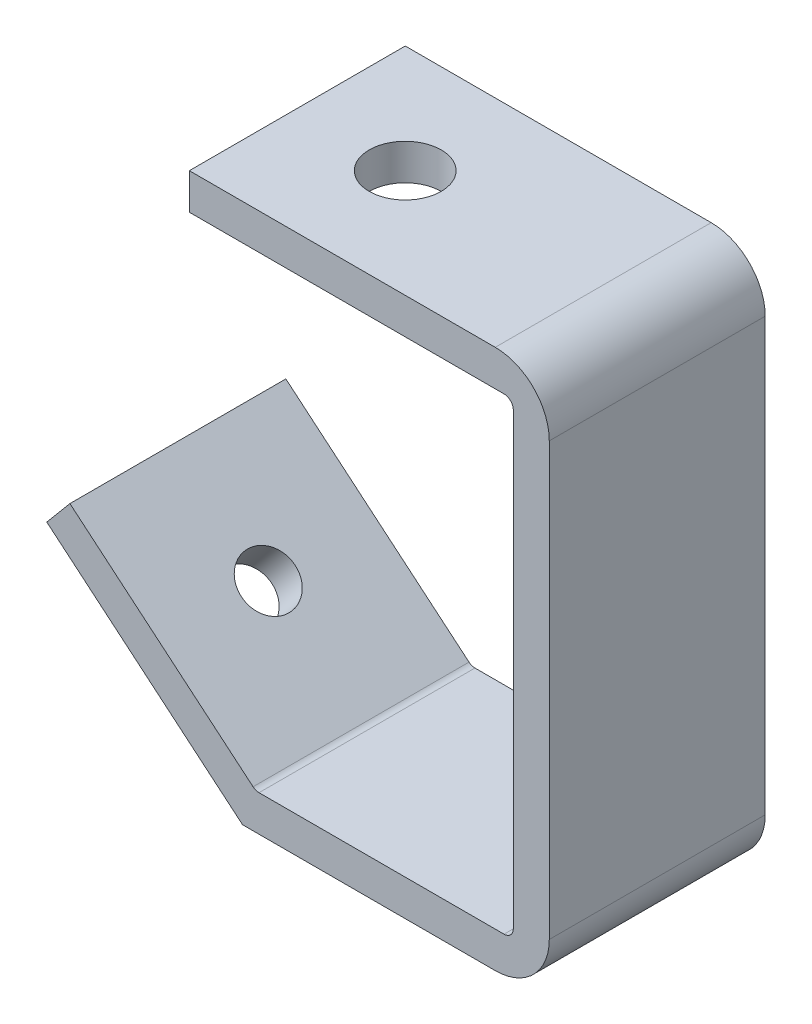
ISO-10303-21;
HEADER;
FILE_DESCRIPTION(('STEP AP214'),'2;1');
FILE_NAME('part.step','',(''),(''),'','','');
FILE_SCHEMA(('AUTOMOTIVE_DESIGN { 1 0 10303 214 1 1 1 1 }'));
ENDSEC;
DATA;
#1=APPLICATION_CONTEXT('core data for automotive mechanical design processes');
#2=APPLICATION_PROTOCOL_DEFINITION('international standard','automotive_design',2000,#1);
#3=PRODUCT_CONTEXT('',#1,'mechanical');
#4=PRODUCT('Part','Part','',(#3));
#5=PRODUCT_RELATED_PRODUCT_CATEGORY('part','',(#4));
#6=PRODUCT_DEFINITION_FORMATION('','',#4);
#7=PRODUCT_DEFINITION_CONTEXT('part definition',#1,'design');
#8=PRODUCT_DEFINITION('design','',#6,#7);
#9=PRODUCT_DEFINITION_SHAPE('','',#8);
#10=(LENGTH_UNIT() NAMED_UNIT(*) SI_UNIT(.MILLI.,.METRE.));
#11=(NAMED_UNIT(*) PLANE_ANGLE_UNIT() SI_UNIT($,.RADIAN.));
#12=(NAMED_UNIT(*) SI_UNIT($,.STERADIAN.) SOLID_ANGLE_UNIT());
#13=UNCERTAINTY_MEASURE_WITH_UNIT(LENGTH_MEASURE(1.E-05),#10,'distance_accuracy_value','');
#14=(GEOMETRIC_REPRESENTATION_CONTEXT(3) GLOBAL_UNCERTAINTY_ASSIGNED_CONTEXT((#13)) GLOBAL_UNIT_ASSIGNED_CONTEXT((#10,
#11,#12)) REPRESENTATION_CONTEXT('',''));
#15=CARTESIAN_POINT('',(0.,0.,0.));
#16=DIRECTION('',(0.,0.,1.));
#17=DIRECTION('',(1.,0.,0.));
#18=AXIS2_PLACEMENT_3D('',#15,#16,#17);
#19=CARTESIAN_POINT('',(-34.5409439402347,28.9832933207661,19.05));
#20=DIRECTION('',(0.64278760968654,0.766044443118977,0.));
#21=DIRECTION('',(-0.766044443118977,0.64278760968654,0.));
#22=AXIS2_PLACEMENT_3D('',#19,#20,#21);
#23=PLANE('',#22);
#24=CARTESIAN_POINT('',(-18.5995590789288,15.6068831631892,0.));
#25=DIRECTION('',(0.64278760968654,0.766044443118977,0.));
#26=DIRECTION('',(-0.766044443118977,0.64278760968654,0.));
#27=AXIS2_PLACEMENT_3D('',#24,#25,#26);
#28=CIRCLE('',#27,4.765);
#29=CARTESIAN_POINT('',(-22.2497608503907,18.6697661233456,0.));
#30=VERTEX_POINT('',#29);
#31=EDGE_CURVE('E185',#30,#30,#28,.T.);
#32=ORIENTED_EDGE('',*,*,#31,.T.);
#33=EDGE_LOOP('',(#32));
#34=FACE_BOUND('',#33,.T.);
#35=DIRECTION('',(0.766044443118977,-0.64278760968654,0.));
#36=VECTOR('',#35,1.);
#37=CARTESIAN_POINT('',(-34.5409439402347,28.9832933207661,-19.05));
#38=LINE('',#37,#36);
#39=CARTESIAN_POINT('',(-34.5409439402347,28.9832933207661,-19.05));
#40=VERTEX_POINT('',#39);
#41=CARTESIAN_POINT('',(0.,0.,-19.05));
#42=VERTEX_POINT('',#41);
#43=EDGE_CURVE('E169',#40,#42,#38,.T.);
#44=ORIENTED_EDGE('',*,*,#43,.T.);
#45=DIRECTION('',(0.,0.,-1.));
#46=VECTOR('',#45,1.);
#47=CARTESIAN_POINT('',(0.,0.,19.05));
#48=LINE('',#47,#46);
#49=CARTESIAN_POINT('',(0.,0.,19.05));
#50=VERTEX_POINT('',#49);
#51=EDGE_CURVE('E148',#50,#42,#48,.T.);
#52=ORIENTED_EDGE('',*,*,#51,.F.);
#53=DIRECTION('',(0.766044443118977,-0.64278760968654,0.));
#54=VECTOR('',#53,1.);
#55=CARTESIAN_POINT('',(-34.5409439402347,28.9832933207661,19.05));
#56=LINE('',#55,#54);
#57=CARTESIAN_POINT('',(-34.5409439402347,28.9832933207661,19.05));
#58=VERTEX_POINT('',#57);
#59=EDGE_CURVE('E157',#58,#50,#56,.T.);
#60=ORIENTED_EDGE('',*,*,#59,.F.);
#61=DIRECTION('',(0.,0.,-1.));
#62=VECTOR('',#61,1.);
#63=CARTESIAN_POINT('',(-34.5409439402347,28.9832933207661,19.05));
#64=LINE('',#63,#62);
#65=EDGE_CURVE('E224',#58,#40,#64,.T.);
#66=ORIENTED_EDGE('',*,*,#65,.T.);
#67=EDGE_LOOP('',(#44,#52,#60,#66));
#68=FACE_BOUND('',#67,.T.);
#69=ADVANCED_FACE('F39',(#34,#68),#23,.F.);
#70=CARTESIAN_POINT('',(0.,0.,19.05));
#71=DIRECTION('',(0.,1.,0.));
#72=DIRECTION('',(0.,0.,1.));
#73=AXIS2_PLACEMENT_3D('',#70,#71,#72);
#74=PLANE('',#73);
#75=DIRECTION('',(1.,0.,0.));
#76=VECTOR('',#75,1.);
#77=CARTESIAN_POINT('',(0.,0.,-19.05));
#78=LINE('',#77,#76);
#79=CARTESIAN_POINT('',(44.5899999999999,0.,-19.05));
#80=VERTEX_POINT('',#79);
#81=EDGE_CURVE('E257',#42,#80,#78,.T.);
#82=ORIENTED_EDGE('',*,*,#81,.T.);
#83=DIRECTION('',(0.,0.,-1.));
#84=VECTOR('',#83,1.);
#85=CARTESIAN_POINT('',(44.5899999999999,0.,19.05));
#86=LINE('',#85,#84);
#87=CARTESIAN_POINT('',(44.5899999999999,0.,19.05));
#88=VERTEX_POINT('',#87);
#89=EDGE_CURVE('E153',#88,#80,#86,.T.);
#90=ORIENTED_EDGE('',*,*,#89,.F.);
#91=DIRECTION('',(1.,0.,0.));
#92=VECTOR('',#91,1.);
#93=CARTESIAN_POINT('',(0.,0.,19.05));
#94=LINE('',#93,#92);
#95=EDGE_CURVE('E147',#50,#88,#94,.T.);
#96=ORIENTED_EDGE('',*,*,#95,.F.);
#97=ORIENTED_EDGE('',*,*,#51,.T.);
#98=EDGE_LOOP('',(#82,#90,#96,#97));
#99=FACE_BOUND('',#98,.T.);
#100=ADVANCED_FACE('F149',(#99),#74,.F.);
#101=CARTESIAN_POINT('',(44.59,9.53,19.05));
#102=DIRECTION('',(0.,0.,-1.));
#103=DIRECTION('',(-1.,0.,0.));
#104=AXIS2_PLACEMENT_3D('',#101,#102,#103);
#105=CYLINDRICAL_SURFACE('',#104,9.53);
#106=CARTESIAN_POINT('',(44.59,9.53,-19.05));
#107=DIRECTION('',(0.,0.,1.));
#108=DIRECTION('',(-1.,0.,0.));
#109=AXIS2_PLACEMENT_3D('',#106,#107,#108);
#110=CIRCLE('',#109,9.53);
#111=CARTESIAN_POINT('',(54.12,9.53000000000007,-19.05));
#112=VERTEX_POINT('',#111);
#113=EDGE_CURVE('E249',#80,#112,#110,.T.);
#114=ORIENTED_EDGE('',*,*,#113,.T.);
#115=DIRECTION('',(0.,0.,-1.));
#116=VECTOR('',#115,1.);
#117=CARTESIAN_POINT('',(54.12,9.53000000000007,19.05));
#118=LINE('',#117,#116);
#119=CARTESIAN_POINT('',(54.12,9.53000000000007,19.05));
#120=VERTEX_POINT('',#119);
#121=EDGE_CURVE('E172',#120,#112,#118,.T.);
#122=ORIENTED_EDGE('',*,*,#121,.F.);
#123=CARTESIAN_POINT('',(44.59,9.53,19.05));
#124=DIRECTION('',(0.,0.,1.));
#125=DIRECTION('',(-1.,0.,0.));
#126=AXIS2_PLACEMENT_3D('',#123,#124,#125);
#127=CIRCLE('',#126,9.53);
#128=EDGE_CURVE('E156',#88,#120,#127,.T.);
#129=ORIENTED_EDGE('',*,*,#128,.F.);
#130=ORIENTED_EDGE('',*,*,#89,.T.);
#131=EDGE_LOOP('',(#114,#122,#129,#130));
#132=FACE_BOUND('',#131,.T.);
#133=ADVANCED_FACE('F287',(#132),#105,.T.);
#134=CARTESIAN_POINT('',(54.12,9.53000000000007,19.05));
#135=DIRECTION('',(-1.,0.,0.));
#136=DIRECTION('',(0.,0.,1.));
#137=AXIS2_PLACEMENT_3D('',#134,#135,#136);
#138=PLANE('',#137);
#139=DIRECTION('',(0.,1.,0.));
#140=VECTOR('',#139,1.);
#141=CARTESIAN_POINT('',(54.12,9.53000000000007,-19.05));
#142=LINE('',#141,#140);
#143=CARTESIAN_POINT('',(54.12,85.7199999999999,-19.05));
#144=VERTEX_POINT('',#143);
#145=EDGE_CURVE('E244',#112,#144,#142,.T.);
#146=ORIENTED_EDGE('',*,*,#145,.T.);
#147=DIRECTION('',(0.,0.,-1.));
#148=VECTOR('',#147,1.);
#149=CARTESIAN_POINT('',(54.12,85.7199999999999,19.05));
#150=LINE('',#149,#148);
#151=CARTESIAN_POINT('',(54.12,85.7199999999999,19.05));
#152=VERTEX_POINT('',#151);
#153=EDGE_CURVE('E236',#152,#144,#150,.T.);
#154=ORIENTED_EDGE('',*,*,#153,.F.);
#155=DIRECTION('',(0.,1.,0.));
#156=VECTOR('',#155,1.);
#157=CARTESIAN_POINT('',(54.12,9.53000000000007,19.05));
#158=LINE('',#157,#156);
#159=EDGE_CURVE('E246',#120,#152,#158,.T.);
#160=ORIENTED_EDGE('',*,*,#159,.F.);
#161=ORIENTED_EDGE('',*,*,#121,.T.);
#162=EDGE_LOOP('',(#146,#154,#160,#161));
#163=FACE_BOUND('',#162,.T.);
#164=ADVANCED_FACE('F243',(#163),#138,.F.);
#165=CARTESIAN_POINT('',(44.59,85.72,19.05));
#166=DIRECTION('',(0.,0.,-1.));
#167=DIRECTION('',(-1.,0.,0.));
#168=AXIS2_PLACEMENT_3D('',#165,#166,#167);
#169=CYLINDRICAL_SURFACE('',#168,9.53);
#170=CARTESIAN_POINT('',(44.59,85.72,-19.05));
#171=DIRECTION('',(0.,0.,1.));
#172=DIRECTION('',(1.,0.,0.));
#173=AXIS2_PLACEMENT_3D('',#170,#171,#172);
#174=CIRCLE('',#173,9.53);
#175=CARTESIAN_POINT('',(44.5899999999999,95.25,-19.05));
#176=VERTEX_POINT('',#175);
#177=EDGE_CURVE('E255',#144,#176,#174,.T.);
#178=ORIENTED_EDGE('',*,*,#177,.T.);
#179=DIRECTION('',(0.,0.,-1.));
#180=VECTOR('',#179,1.);
#181=CARTESIAN_POINT('',(44.5899999999999,95.25,19.05));
#182=LINE('',#181,#180);
#183=CARTESIAN_POINT('',(44.5899999999999,95.25,19.05));
#184=VERTEX_POINT('',#183);
#185=EDGE_CURVE('E231',#184,#176,#182,.T.);
#186=ORIENTED_EDGE('',*,*,#185,.F.);
#187=CARTESIAN_POINT('',(44.59,85.72,19.05));
#188=DIRECTION('',(0.,0.,1.));
#189=DIRECTION('',(1.,0.,0.));
#190=AXIS2_PLACEMENT_3D('',#187,#188,#189);
#191=CIRCLE('',#190,9.53);
#192=EDGE_CURVE('E288',#152,#184,#191,.T.);
#193=ORIENTED_EDGE('',*,*,#192,.F.);
#194=ORIENTED_EDGE('',*,*,#153,.T.);
#195=EDGE_LOOP('',(#178,#186,#193,#194));
#196=FACE_BOUND('',#195,.T.);
#197=ADVANCED_FACE('F320',(#196),#169,.T.);
#198=CARTESIAN_POINT('',(44.5899999999999,95.25,19.05));
#199=DIRECTION('',(0.,-1.,0.));
#200=DIRECTION('',(1.,0.,0.));
#201=AXIS2_PLACEMENT_3D('',#198,#199,#200);
#202=PLANE('',#201);
#203=CARTESIAN_POINT('',(9.64999999999999,95.25,0.));
#204=DIRECTION('',(0.,-1.,0.));
#205=DIRECTION('',(1.,0.,0.));
#206=AXIS2_PLACEMENT_3D('',#203,#204,#205);
#207=CIRCLE('',#206,6.35);
#208=CARTESIAN_POINT('',(3.29999999999999,95.25,0.));
#209=VERTEX_POINT('',#208);
#210=EDGE_CURVE('E181',#209,#209,#207,.T.);
#211=ORIENTED_EDGE('',*,*,#210,.T.);
#212=EDGE_LOOP('',(#211));
#213=FACE_BOUND('',#212,.T.);
#214=DIRECTION('',(-1.,0.,0.));
#215=VECTOR('',#214,1.);
#216=CARTESIAN_POINT('',(44.5899999999999,95.25,-19.05));
#217=LINE('',#216,#215);
#218=CARTESIAN_POINT('',(-9.39,95.25,-19.05));
#219=VERTEX_POINT('',#218);
#220=EDGE_CURVE('E251',#176,#219,#217,.T.);
#221=ORIENTED_EDGE('',*,*,#220,.T.);
#222=DIRECTION('',(0.,0.,-1.));
#223=VECTOR('',#222,1.);
#224=CARTESIAN_POINT('',(-9.39,95.25,19.05));
#225=LINE('',#224,#223);
#226=CARTESIAN_POINT('',(-9.39,95.25,19.05));
#227=VERTEX_POINT('',#226);
#228=EDGE_CURVE('E229',#227,#219,#225,.T.);
#229=ORIENTED_EDGE('',*,*,#228,.F.);
#230=DIRECTION('',(-1.,0.,0.));
#231=VECTOR('',#230,1.);
#232=CARTESIAN_POINT('',(44.5899999999999,95.25,19.05));
#233=LINE('',#232,#231);
#234=EDGE_CURVE('E291',#184,#227,#233,.T.);
#235=ORIENTED_EDGE('',*,*,#234,.F.);
#236=ORIENTED_EDGE('',*,*,#185,.T.);
#237=EDGE_LOOP('',(#221,#229,#235,#236));
#238=FACE_BOUND('',#237,.T.);
#239=ADVANCED_FACE('F315',(#213,#238),#202,.F.);
#240=CARTESIAN_POINT('',(-9.39,95.25,19.05));
#241=DIRECTION('',(1.,0.,0.));
#242=DIRECTION('',(0.,0.,-1.));
#243=AXIS2_PLACEMENT_3D('',#240,#241,#242);
#244=PLANE('',#243);
#245=DIRECTION('',(0.,-1.,0.));
#246=VECTOR('',#245,1.);
#247=CARTESIAN_POINT('',(-9.39,95.25,-19.05));
#248=LINE('',#247,#246);
#249=CARTESIAN_POINT('',(-9.39,88.9,-19.05));
#250=VERTEX_POINT('',#249);
#251=EDGE_CURVE('E261',#219,#250,#248,.T.);
#252=ORIENTED_EDGE('',*,*,#251,.T.);
#253=DIRECTION('',(0.,0.,-1.));
#254=VECTOR('',#253,1.);
#255=CARTESIAN_POINT('',(-9.39,88.9,19.05));
#256=LINE('',#255,#254);
#257=CARTESIAN_POINT('',(-9.39,88.9,19.05));
#258=VERTEX_POINT('',#257);
#259=EDGE_CURVE('E227',#258,#250,#256,.T.);
#260=ORIENTED_EDGE('',*,*,#259,.F.);
#261=DIRECTION('',(0.,-1.,0.));
#262=VECTOR('',#261,1.);
#263=CARTESIAN_POINT('',(-9.39,95.25,19.05));
#264=LINE('',#263,#262);
#265=EDGE_CURVE('E294',#227,#258,#264,.T.);
#266=ORIENTED_EDGE('',*,*,#265,.F.);
#267=ORIENTED_EDGE('',*,*,#228,.T.);
#268=EDGE_LOOP('',(#252,#260,#266,#267));
#269=FACE_BOUND('',#268,.T.);
#270=ADVANCED_FACE('F307',(#269),#244,.F.);
#271=CARTESIAN_POINT('',(-9.39,88.9,19.05));
#272=DIRECTION('',(0.,1.,0.));
#273=DIRECTION('',(0.,0.,1.));
#274=AXIS2_PLACEMENT_3D('',#271,#272,#273);
#275=PLANE('',#274);
#276=CARTESIAN_POINT('',(9.65,88.9,0.));
#277=DIRECTION('',(0.,1.,0.));
#278=DIRECTION('',(0.,0.,1.));
#279=AXIS2_PLACEMENT_3D('',#276,#277,#278);
#280=CIRCLE('',#279,6.35);
#281=CARTESIAN_POINT('',(3.3,88.9,0.));
#282=VERTEX_POINT('',#281);
#283=EDGE_CURVE('E178',#282,#282,#280,.T.);
#284=ORIENTED_EDGE('',*,*,#283,.T.);
#285=EDGE_LOOP('',(#284));
#286=FACE_BOUND('',#285,.T.);
#287=DIRECTION('',(1.,0.,0.));
#288=VECTOR('',#287,1.);
#289=CARTESIAN_POINT('',(-9.39,88.9,-19.05));
#290=LINE('',#289,#288);
#291=CARTESIAN_POINT('',(46.14,88.9,-19.05));
#292=VERTEX_POINT('',#291);
#293=EDGE_CURVE('E263',#250,#292,#290,.T.);
#294=ORIENTED_EDGE('',*,*,#293,.T.);
#295=DIRECTION('',(0.,0.,-1.));
#296=VECTOR('',#295,1.);
#297=CARTESIAN_POINT('',(46.14,88.9,19.05));
#298=LINE('',#297,#296);
#299=CARTESIAN_POINT('',(46.14,88.9,19.05));
#300=VERTEX_POINT('',#299);
#301=EDGE_CURVE('E189',#292,#300,#298,.F.);
#302=ORIENTED_EDGE('',*,*,#301,.T.);
#303=DIRECTION('',(1.,0.,0.));
#304=VECTOR('',#303,1.);
#305=CARTESIAN_POINT('',(-9.39,88.9,19.05));
#306=LINE('',#305,#304);
#307=EDGE_CURVE('E285',#258,#300,#306,.T.);
#308=ORIENTED_EDGE('',*,*,#307,.F.);
#309=ORIENTED_EDGE('',*,*,#259,.T.);
#310=EDGE_LOOP('',(#294,#302,#308,#309));
#311=FACE_BOUND('',#310,.T.);
#312=ADVANCED_FACE('F310',(#286,#311),#275,.F.);
#313=CARTESIAN_POINT('',(47.77,88.9,19.05));
#314=DIRECTION('',(1.,0.,0.));
#315=DIRECTION('',(0.,1.,0.));
#316=AXIS2_PLACEMENT_3D('',#313,#314,#315);
#317=PLANE('',#316);
#318=DIRECTION('',(0.,-1.,0.));
#319=VECTOR('',#318,1.);
#320=CARTESIAN_POINT('',(47.77,88.9,19.05));
#321=LINE('',#320,#319);
#322=CARTESIAN_POINT('',(47.77,87.27,19.05));
#323=VERTEX_POINT('',#322);
#324=CARTESIAN_POINT('',(47.77,7.98,19.05));
#325=VERTEX_POINT('',#324);
#326=EDGE_CURVE('E279',#323,#325,#321,.T.);
#327=ORIENTED_EDGE('',*,*,#326,.F.);
#328=DIRECTION('',(0.,0.,-1.));
#329=VECTOR('',#328,1.);
#330=CARTESIAN_POINT('',(47.77,87.27,-19.05));
#331=LINE('',#330,#329);
#332=CARTESIAN_POINT('',(47.77,87.27,-19.05));
#333=VERTEX_POINT('',#332);
#334=EDGE_CURVE('E175',#323,#333,#331,.T.);
#335=ORIENTED_EDGE('',*,*,#334,.T.);
#336=DIRECTION('',(0.,-1.,0.));
#337=VECTOR('',#336,1.);
#338=CARTESIAN_POINT('',(47.77,88.9,-19.05));
#339=LINE('',#338,#337);
#340=CARTESIAN_POINT('',(47.77,7.98,-19.05));
#341=VERTEX_POINT('',#340);
#342=EDGE_CURVE('E217',#333,#341,#339,.T.);
#343=ORIENTED_EDGE('',*,*,#342,.T.);
#344=DIRECTION('',(0.,0.,-1.));
#345=VECTOR('',#344,1.);
#346=CARTESIAN_POINT('',(47.77,7.98,19.05));
#347=LINE('',#346,#345);
#348=EDGE_CURVE('E167',#341,#325,#347,.F.);
#349=ORIENTED_EDGE('',*,*,#348,.T.);
#350=EDGE_LOOP('',(#327,#335,#343,#349));
#351=FACE_BOUND('',#350,.T.);
#352=ADVANCED_FACE('F270',(#351),#317,.F.);
#353=CARTESIAN_POINT('',(47.77,6.35,19.05));
#354=DIRECTION('',(0.,-1.,0.));
#355=DIRECTION('',(1.,0.,0.));
#356=AXIS2_PLACEMENT_3D('',#353,#354,#355);
#357=PLANE('',#356);
#358=DIRECTION('',(-1.,0.,0.));
#359=VECTOR('',#358,1.);
#360=CARTESIAN_POINT('',(47.77,6.35,-19.05));
#361=LINE('',#360,#359);
#362=CARTESIAN_POINT('',(46.14,6.35,-19.05));
#363=VERTEX_POINT('',#362);
#364=CARTESIAN_POINT('',(2.90448246944432,6.35,-19.05));
#365=VERTEX_POINT('',#364);
#366=EDGE_CURVE('E216',#363,#365,#361,.T.);
#367=ORIENTED_EDGE('',*,*,#366,.T.);
#368=DIRECTION('',(0.,0.,-1.));
#369=VECTOR('',#368,1.);
#370=CARTESIAN_POINT('',(2.90448246944432,6.35,19.05));
#371=LINE('',#370,#369);
#372=CARTESIAN_POINT('',(2.90448246944432,6.35,19.05));
#373=VERTEX_POINT('',#372);
#374=EDGE_CURVE('E58',#365,#373,#371,.F.);
#375=ORIENTED_EDGE('',*,*,#374,.T.);
#376=DIRECTION('',(-1.,0.,0.));
#377=VECTOR('',#376,1.);
#378=CARTESIAN_POINT('',(47.77,6.35,19.05));
#379=LINE('',#378,#377);
#380=CARTESIAN_POINT('',(46.14,6.35,19.05));
#381=VERTEX_POINT('',#380);
#382=EDGE_CURVE('E280',#381,#373,#379,.T.);
#383=ORIENTED_EDGE('',*,*,#382,.F.);
#384=DIRECTION('',(0.,0.,-1.));
#385=VECTOR('',#384,1.);
#386=CARTESIAN_POINT('',(46.14,6.35,-19.05));
#387=LINE('',#386,#385);
#388=EDGE_CURVE('E188',#381,#363,#387,.T.);
#389=ORIENTED_EDGE('',*,*,#388,.T.);
#390=EDGE_LOOP('',(#367,#375,#383,#389));
#391=FACE_BOUND('',#390,.T.);
#392=ADVANCED_FACE('F276',(#391),#357,.F.);
#393=CARTESIAN_POINT('',(2.31121098759041,6.35,19.05));
#394=DIRECTION('',(-0.64278760968654,-0.766044443118977,0.));
#395=DIRECTION('',(0.766044443118977,-0.64278760968654,0.));
#396=AXIS2_PLACEMENT_3D('',#393,#394,#395);
#397=PLANE('',#396);
#398=CARTESIAN_POINT('',(-14.5178577574192,20.4712653769947,0.));
#399=DIRECTION('',(-0.64278760968654,-0.766044443118977,0.));
#400=DIRECTION('',(0.766044443118977,-0.64278760968654,0.));
#401=AXIS2_PLACEMENT_3D('',#398,#399,#400);
#402=CIRCLE('',#401,4.765);
#403=CARTESIAN_POINT('',(-10.8676559859573,17.4083824168383,0.));
#404=VERTEX_POINT('',#403);
#405=EDGE_CURVE('E182',#404,#404,#402,.T.);
#406=ORIENTED_EDGE('',*,*,#405,.T.);
#407=EDGE_LOOP('',(#406));
#408=FACE_BOUND('',#407,.T.);
#409=DIRECTION('',(-0.766044443118977,0.64278760968654,0.));
#410=VECTOR('',#409,1.);
#411=CARTESIAN_POINT('',(2.31121098759041,6.35,19.05));
#412=LINE('',#411,#410);
#413=CARTESIAN_POINT('',(1.85673866565526,6.73134755771606,19.05));
#414=VERTEX_POINT('',#413);
#415=CARTESIAN_POINT('',(-30.4592426187252,33.8476755345716,19.05));
#416=VERTEX_POINT('',#415);
#417=EDGE_CURVE('E212',#414,#416,#412,.T.);
#418=ORIENTED_EDGE('',*,*,#417,.F.);
#419=DIRECTION('',(0.,0.,-1.));
#420=VECTOR('',#419,1.);
#421=CARTESIAN_POINT('',(1.85673866565526,6.73134755771606,-19.05));
#422=LINE('',#421,#420);
#423=CARTESIAN_POINT('',(1.85673866565526,6.73134755771606,-19.05));
#424=VERTEX_POINT('',#423);
#425=EDGE_CURVE('E201',#414,#424,#422,.T.);
#426=ORIENTED_EDGE('',*,*,#425,.T.);
#427=DIRECTION('',(-0.766044443118977,0.64278760968654,0.));
#428=VECTOR('',#427,1.);
#429=CARTESIAN_POINT('',(2.31121098759041,6.35,-19.05));
#430=LINE('',#429,#428);
#431=CARTESIAN_POINT('',(-30.4592426187252,33.8476755345716,-19.05));
#432=VERTEX_POINT('',#431);
#433=EDGE_CURVE('E209',#424,#432,#430,.T.);
#434=ORIENTED_EDGE('',*,*,#433,.T.);
#435=DIRECTION('',(0.,0.,-1.));
#436=VECTOR('',#435,1.);
#437=CARTESIAN_POINT('',(-30.4592426187252,33.8476755345716,19.05));
#438=LINE('',#437,#436);
#439=EDGE_CURVE('E225',#416,#432,#438,.T.);
#440=ORIENTED_EDGE('',*,*,#439,.F.);
#441=EDGE_LOOP('',(#418,#426,#434,#440));
#442=FACE_BOUND('',#441,.T.);
#443=ADVANCED_FACE('F210',(#408,#442),#397,.F.);
#444=CARTESIAN_POINT('',(-30.4592426187252,33.8476755345716,19.05));
#445=DIRECTION('',(0.766044443118978,-0.642787609686539,0.));
#446=DIRECTION('',(0.642787609686539,0.766044443118978,0.));
#447=AXIS2_PLACEMENT_3D('',#444,#445,#446);
#448=PLANE('',#447);
#449=DIRECTION('',(-0.642787609686539,-0.766044443118978,0.));
#450=VECTOR('',#449,1.);
#451=CARTESIAN_POINT('',(-30.4592426187252,33.8476755345716,-19.05));
#452=LINE('',#451,#450);
#453=EDGE_CURVE('E168',#432,#40,#452,.T.);
#454=ORIENTED_EDGE('',*,*,#453,.T.);
#455=ORIENTED_EDGE('',*,*,#65,.F.);
#456=DIRECTION('',(-0.642787609686539,-0.766044443118978,0.));
#457=VECTOR('',#456,1.);
#458=CARTESIAN_POINT('',(-30.4592426187252,33.8476755345716,19.05));
#459=LINE('',#458,#457);
#460=EDGE_CURVE('E162',#416,#58,#459,.T.);
#461=ORIENTED_EDGE('',*,*,#460,.F.);
#462=ORIENTED_EDGE('',*,*,#439,.T.);
#463=EDGE_LOOP('',(#454,#455,#461,#462));
#464=FACE_BOUND('',#463,.T.);
#465=ADVANCED_FACE('F351',(#464),#448,.F.);
#466=CARTESIAN_POINT('',(44.59,9.53,19.05));
#467=DIRECTION('',(0.,0.,-1.));
#468=DIRECTION('',(-1.,0.,0.));
#469=AXIS2_PLACEMENT_3D('',#466,#467,#468);
#470=PLANE('',#469);
#471=ORIENTED_EDGE('',*,*,#59,.T.);
#472=ORIENTED_EDGE('',*,*,#95,.T.);
#473=ORIENTED_EDGE('',*,*,#128,.T.);
#474=ORIENTED_EDGE('',*,*,#159,.T.);
#475=ORIENTED_EDGE('',*,*,#192,.T.);
#476=ORIENTED_EDGE('',*,*,#234,.T.);
#477=ORIENTED_EDGE('',*,*,#265,.T.);
#478=ORIENTED_EDGE('',*,*,#307,.T.);
#479=CARTESIAN_POINT('',(46.14,87.27,19.05));
#480=DIRECTION('',(0.,0.,-1.));
#481=DIRECTION('',(-1.,0.,0.));
#482=AXIS2_PLACEMENT_3D('',#479,#480,#481);
#483=CIRCLE('',#482,1.63);
#484=EDGE_CURVE('E193',#300,#323,#483,.T.);
#485=ORIENTED_EDGE('',*,*,#484,.T.);
#486=ORIENTED_EDGE('',*,*,#326,.T.);
#487=CARTESIAN_POINT('',(46.14,7.98,19.05));
#488=DIRECTION('',(0.,0.,-1.));
#489=DIRECTION('',(-1.,0.,0.));
#490=AXIS2_PLACEMENT_3D('',#487,#488,#489);
#491=CIRCLE('',#490,1.63);
#492=EDGE_CURVE('E197',#325,#381,#491,.T.);
#493=ORIENTED_EDGE('',*,*,#492,.T.);
#494=ORIENTED_EDGE('',*,*,#382,.T.);
#495=CARTESIAN_POINT('',(2.90448246944432,7.98,19.05));
#496=DIRECTION('',(0.,0.,-1.));
#497=DIRECTION('',(-1.,0.,0.));
#498=AXIS2_PLACEMENT_3D('',#495,#496,#497);
#499=CIRCLE('',#498,1.63);
#500=EDGE_CURVE('E11',#373,#414,#499,.T.);
#501=ORIENTED_EDGE('',*,*,#500,.T.);
#502=ORIENTED_EDGE('',*,*,#417,.T.);
#503=ORIENTED_EDGE('',*,*,#460,.T.);
#504=EDGE_LOOP('',(#471,#472,#473,#474,#475,#476,#477,#478,#485,#486,#493,#494,#501,#502,#503));
#505=FACE_BOUND('',#504,.T.);
#506=ADVANCED_FACE('F160',(#505),#470,.F.);
#507=CARTESIAN_POINT('',(44.59,9.53,-19.05));
#508=DIRECTION('',(0.,0.,-1.));
#509=DIRECTION('',(-1.,0.,0.));
#510=AXIS2_PLACEMENT_3D('',#507,#508,#509);
#511=PLANE('',#510);
#512=ORIENTED_EDGE('',*,*,#43,.F.);
#513=ORIENTED_EDGE('',*,*,#453,.F.);
#514=ORIENTED_EDGE('',*,*,#433,.F.);
#515=CARTESIAN_POINT('',(2.90448246944432,7.98,-19.05));
#516=DIRECTION('',(0.,0.,-1.));
#517=DIRECTION('',(-1.,0.,0.));
#518=AXIS2_PLACEMENT_3D('',#515,#516,#517);
#519=CIRCLE('',#518,1.63);
#520=EDGE_CURVE('E50',#424,#365,#519,.F.);
#521=ORIENTED_EDGE('',*,*,#520,.T.);
#522=ORIENTED_EDGE('',*,*,#366,.F.);
#523=CARTESIAN_POINT('',(46.14,7.98,-19.05));
#524=DIRECTION('',(0.,0.,-1.));
#525=DIRECTION('',(-1.,0.,0.));
#526=AXIS2_PLACEMENT_3D('',#523,#524,#525);
#527=CIRCLE('',#526,1.63);
#528=EDGE_CURVE('E200',#363,#341,#527,.F.);
#529=ORIENTED_EDGE('',*,*,#528,.T.);
#530=ORIENTED_EDGE('',*,*,#342,.F.);
#531=CARTESIAN_POINT('',(46.14,87.27,-19.05));
#532=DIRECTION('',(0.,0.,-1.));
#533=DIRECTION('',(-1.,0.,0.));
#534=AXIS2_PLACEMENT_3D('',#531,#532,#533);
#535=CIRCLE('',#534,1.63);
#536=EDGE_CURVE('E194',#333,#292,#535,.F.);
#537=ORIENTED_EDGE('',*,*,#536,.T.);
#538=ORIENTED_EDGE('',*,*,#293,.F.);
#539=ORIENTED_EDGE('',*,*,#251,.F.);
#540=ORIENTED_EDGE('',*,*,#220,.F.);
#541=ORIENTED_EDGE('',*,*,#177,.F.);
#542=ORIENTED_EDGE('',*,*,#145,.F.);
#543=ORIENTED_EDGE('',*,*,#113,.F.);
#544=ORIENTED_EDGE('',*,*,#81,.F.);
#545=EDGE_LOOP('',(#512,#513,#514,#521,#522,#529,#530,#537,#538,#539,#540,#541,#542,#543,#544));
#546=FACE_BOUND('',#545,.T.);
#547=ADVANCED_FACE('F213',(#546),#511,.T.);
#548=CARTESIAN_POINT('',(9.65,76.2,0.));
#549=DIRECTION('',(0.,1.,0.));
#550=DIRECTION('',(-1.,0.,0.));
#551=AXIS2_PLACEMENT_3D('',#548,#549,#550);
#552=CYLINDRICAL_SURFACE('',#551,6.35);
#553=CARTESIAN_POINT('',(3.3,88.9,0.));
#554=CARTESIAN_POINT('',(3.3,88.9661458333333,0.));
#555=CARTESIAN_POINT('',(3.3,89.0322916666667,0.));
#556=CARTESIAN_POINT('',(3.3,89.1645833333333,0.));
#557=CARTESIAN_POINT('',(3.3,89.2307291666667,0.));
#558=CARTESIAN_POINT('',(3.3,89.3630208333333,0.));
#559=CARTESIAN_POINT('',(3.3,89.4291666666667,0.));
#560=CARTESIAN_POINT('',(3.3,89.5614583333333,0.));
#561=CARTESIAN_POINT('',(3.3,89.6276041666667,0.));
#562=CARTESIAN_POINT('',(3.3,89.7598958333333,0.));
#563=CARTESIAN_POINT('',(3.3,89.8260416666667,0.));
#564=CARTESIAN_POINT('',(3.3,89.9583333333333,0.));
#565=CARTESIAN_POINT('',(3.3,90.0244791666667,0.));
#566=CARTESIAN_POINT('',(3.3,90.1567708333333,0.));
#567=CARTESIAN_POINT('',(3.3,90.2229166666666,0.));
#568=CARTESIAN_POINT('',(3.3,90.3552083333333,0.));
#569=CARTESIAN_POINT('',(3.3,90.4213541666666,0.));
#570=CARTESIAN_POINT('',(3.3,90.5536458333333,0.));
#571=CARTESIAN_POINT('',(3.3,90.6197916666667,0.));
#572=CARTESIAN_POINT('',(3.3,90.7520833333333,0.));
#573=CARTESIAN_POINT('',(3.3,90.8182291666667,0.));
#574=CARTESIAN_POINT('',(3.3,90.9505208333333,0.));
#575=CARTESIAN_POINT('',(3.3,91.0166666666667,0.));
#576=CARTESIAN_POINT('',(3.3,91.1489583333333,0.));
#577=CARTESIAN_POINT('',(3.3,91.2151041666666,0.));
#578=CARTESIAN_POINT('',(3.3,91.3473958333333,0.));
#579=CARTESIAN_POINT('',(3.3,91.4135416666667,0.));
#580=CARTESIAN_POINT('',(3.3,91.5458333333333,0.));
#581=CARTESIAN_POINT('',(3.3,91.6119791666666,0.));
#582=CARTESIAN_POINT('',(3.3,91.7442708333333,0.));
#583=CARTESIAN_POINT('',(3.3,91.8104166666666,0.));
#584=CARTESIAN_POINT('',(3.3,91.9427083333333,0.));
#585=CARTESIAN_POINT('',(3.3,92.0088541666666,0.));
#586=CARTESIAN_POINT('',(3.3,92.1411458333333,0.));
#587=CARTESIAN_POINT('',(3.3,92.2072916666666,0.));
#588=CARTESIAN_POINT('',(3.3,92.3395833333333,0.));
#589=CARTESIAN_POINT('',(3.3,92.4057291666666,0.));
#590=CARTESIAN_POINT('',(3.3,92.5380208333333,0.));
#591=CARTESIAN_POINT('',(3.3,92.6041666666666,0.));
#592=CARTESIAN_POINT('',(3.3,92.7364583333333,0.));
#593=CARTESIAN_POINT('',(3.3,92.8026041666666,0.));
#594=CARTESIAN_POINT('',(3.3,92.9348958333333,0.));
#595=CARTESIAN_POINT('',(3.3,93.0010416666667,0.));
#596=CARTESIAN_POINT('',(3.3,93.1333333333333,0.));
#597=CARTESIAN_POINT('',(3.3,93.1994791666666,0.));
#598=CARTESIAN_POINT('',(3.3,93.3317708333333,0.));
#599=CARTESIAN_POINT('',(3.3,93.3979166666666,0.));
#600=CARTESIAN_POINT('',(3.3,93.5302083333333,0.));
#601=CARTESIAN_POINT('',(3.3,93.5963541666666,0.));
#602=CARTESIAN_POINT('',(3.3,93.7286458333333,0.));
#603=CARTESIAN_POINT('',(3.3,93.7947916666666,0.));
#604=CARTESIAN_POINT('',(3.3,93.9270833333333,0.));
#605=CARTESIAN_POINT('',(3.3,93.9932291666666,0.));
#606=CARTESIAN_POINT('',(3.3,94.1255208333333,0.));
#607=CARTESIAN_POINT('',(3.3,94.1916666666666,0.));
#608=CARTESIAN_POINT('',(3.3,94.3239583333333,0.));
#609=CARTESIAN_POINT('',(3.29999999999999,94.3901041666666,0.));
#610=CARTESIAN_POINT('',(3.29999999999999,94.5223958333333,0.));
#611=CARTESIAN_POINT('',(3.29999999999999,94.5885416666666,0.));
#612=CARTESIAN_POINT('',(3.29999999999999,94.7208333333333,0.));
#613=CARTESIAN_POINT('',(3.29999999999999,94.7869791666666,0.));
#614=CARTESIAN_POINT('',(3.29999999999999,94.9192708333333,0.));
#615=CARTESIAN_POINT('',(3.29999999999999,94.9854166666666,0.));
#616=CARTESIAN_POINT('',(3.29999999999999,95.1177083333333,0.));
#617=CARTESIAN_POINT('',(3.29999999999999,95.1838541666666,0.));
#618=CARTESIAN_POINT('',(3.29999999999999,95.25,0.));
#619=B_SPLINE_CURVE_WITH_KNOTS('',3,(#553,#554,#555,#556,#557,#558,#559,#560,#561,#562,#563,
#564,#565,#566,#567,#568,#569,#570,#571,#572,#573,#574,#575,#576,#577,#578,#579,#580,#581,#582,
#583,#584,#585,#586,#587,#588,#589,#590,#591,#592,#593,#594,#595,#596,#597,#598,#599,#600,#601,
#602,#603,#604,#605,#606,#607,#608,#609,#610,#611,#612,#613,#614,#615,#616,#617,#618),
.UNSPECIFIED.,.F.,.F.,(4,2,2,2,2,2,2,2,2,2,2,2,2,2,2,2,2,2,2,2,2,2,2,2,2,2,2,2,2,2,2,2,4),(0.,
0.198437500000009,0.396875000000005,0.5953125,0.793749999999996,0.992187500000005,1.190625,
1.3890625,1.58749999999999,1.7859375,1.984375,2.18281249999999,2.38124999999999,2.5796875,
2.77812499999999,2.97656249999999,3.17499999999998,3.37343749999998,3.57187499999999,
3.77031249999998,3.96874999999998,4.16718749999999,4.36562499999998,4.56406249999998,
4.76249999999998,4.96093749999997,5.15937499999998,5.35781249999998,5.55624999999997,
5.75468749999998,5.95312499999998,6.15156249999997,6.34999999999997),.UNSPECIFIED.);
#620=EDGE_CURVE('BSEAM419',#282,#209,#619,.T.);
#621=ORIENTED_EDGE('',*,*,#283,.F.);
#622=ORIENTED_EDGE('',*,*,#210,.F.);
#623=ORIENTED_EDGE('',*,*,#620,.T.);
#624=ORIENTED_EDGE('',*,*,#620,.F.);
#625=EDGE_LOOP('',(#621,#623,#622,#624));
#626=FACE_BOUND('',#625,.T.);
#627=ADVANCED_FACE('F419',(#626),#552,.F.);
#628=CARTESIAN_POINT('',(-6.35445511440018,30.2000298046057,0.));
#629=DIRECTION('',(-0.64278760968654,-0.766044443118977,0.));
#630=DIRECTION('',(0.766044443118977,-0.64278760968654,0.));
#631=AXIS2_PLACEMENT_3D('',#628,#629,#630);
#632=CYLINDRICAL_SURFACE('',#631,4.765);
#633=ORIENTED_EDGE('',*,*,#405,.F.);
#634=EDGE_LOOP('',(#633));
#635=FACE_BOUND('',#634,.T.);
#636=ORIENTED_EDGE('',*,*,#31,.F.);
#637=EDGE_LOOP('',(#636));
#638=FACE_BOUND('',#637,.T.);
#639=ADVANCED_FACE('F342',(#635,#638),#632,.F.);
#640=CARTESIAN_POINT('',(46.14,87.27,19.05));
#641=DIRECTION('',(0.,0.,1.));
#642=DIRECTION('',(1.,0.,0.));
#643=AXIS2_PLACEMENT_3D('',#640,#641,#642);
#644=CYLINDRICAL_SURFACE('',#643,1.63);
#645=ORIENTED_EDGE('',*,*,#484,.F.);
#646=ORIENTED_EDGE('',*,*,#301,.F.);
#647=ORIENTED_EDGE('',*,*,#536,.F.);
#648=ORIENTED_EDGE('',*,*,#334,.F.);
#649=EDGE_LOOP('',(#645,#646,#647,#648));
#650=FACE_BOUND('',#649,.T.);
#651=ADVANCED_FACE('F302',(#650),#644,.F.);
#652=CARTESIAN_POINT('',(46.14,7.98,19.05));
#653=DIRECTION('',(0.,0.,1.));
#654=DIRECTION('',(1.,0.,0.));
#655=AXIS2_PLACEMENT_3D('',#652,#653,#654);
#656=CYLINDRICAL_SURFACE('',#655,1.63);
#657=ORIENTED_EDGE('',*,*,#492,.F.);
#658=ORIENTED_EDGE('',*,*,#348,.F.);
#659=ORIENTED_EDGE('',*,*,#528,.F.);
#660=ORIENTED_EDGE('',*,*,#388,.F.);
#661=EDGE_LOOP('',(#657,#658,#659,#660));
#662=FACE_BOUND('',#661,.T.);
#663=ADVANCED_FACE('F273',(#662),#656,.F.);
#664=CARTESIAN_POINT('',(2.90448246944432,7.98,19.05));
#665=DIRECTION('',(0.,0.,1.));
#666=DIRECTION('',(1.,0.,0.));
#667=AXIS2_PLACEMENT_3D('',#664,#665,#666);
#668=CYLINDRICAL_SURFACE('',#667,1.63);
#669=ORIENTED_EDGE('',*,*,#500,.F.);
#670=ORIENTED_EDGE('',*,*,#374,.F.);
#671=ORIENTED_EDGE('',*,*,#520,.F.);
#672=ORIENTED_EDGE('',*,*,#425,.F.);
#673=EDGE_LOOP('',(#669,#670,#671,#672));
#674=FACE_BOUND('',#673,.T.);
#675=ADVANCED_FACE('F41',(#674),#668,.F.);
#676=CLOSED_SHELL('',(#69,#100,#133,#164,#197,#239,#270,#312,#352,#392,#443,#465,#506,#547,#627,
#639,#651,#663,#675));
#677=MANIFOLD_SOLID_BREP('B2',#676);
#678=ADVANCED_BREP_SHAPE_REPRESENTATION('',(#18,#677),#14);
#679=SHAPE_DEFINITION_REPRESENTATION(#9,#678);
ENDSEC;
END-ISO-10303-21;
